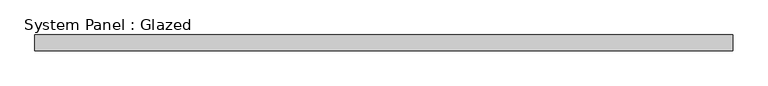
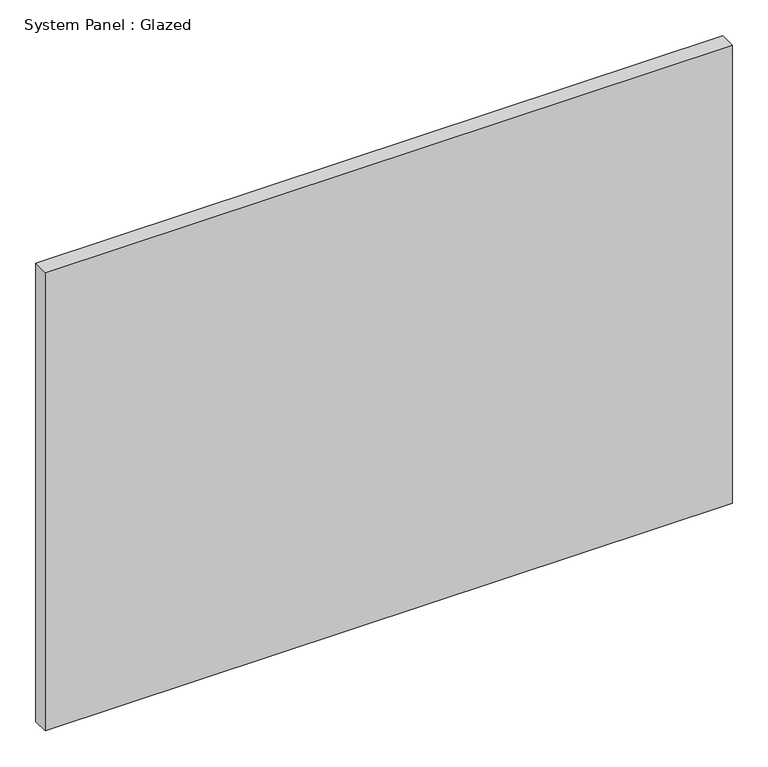
"""IFC4 building model written with IfcOpenShell, lengths in millimetres: plate geometry, System Panel : Glazed."""

from ifc_helpers import new_model, si_unit, origin, origin_with_axes, place, context, project, spatial, polyline, outline, extrude, source, transform, mapped, element, save


def system_panel_glazed_e970100d(model_context):
    return source(origin(), model_context, "Body", "SweptSolid", [
        extrude(outline(polyline([(551.392122, 19.05), (-551.392122, 19.05), (-551.392122, 44.45), (551.392122, 44.45), (551.392122, 19.05)])), origin_with_axes(), (0.0, 0.0, 1.0), 777.5290241),
    ])


if __name__ == "__main__":
    model = new_model("IFC4")
    model_context = context("Model", 3, world=origin())
    ifc_project = project(units=[si_unit("LENGTHUNIT", "METRE", prefix="MILLI")], contexts=[model_context])
    site = spatial("IfcSite", under=ifc_project)
    building = spatial("IfcBuilding", under=site)
    placement = place(None, origin())
    system_panel_glazed_shape = system_panel_glazed_e970100d(model_context)
    element("IfcPlate", 1, ObjectType="System Panel : Glazed", at=placement, inside=building, context=model_context, shape_type="MappedRepresentation", body=[
        mapped(system_panel_glazed_shape, transform((0.0, 0.0, 0.0), x_axis=(1.0, 0.0, 0.0), y_axis=(0.0, 1.0, 0.0), z_axis=(0.0, 0.0, 1.0))),
    ])
    save(model, "model.ifc")

# Revit data of these elements
# Type "System Panel : Glazed"
#   Construction Type Id = "GSP4R"
#   Analytic Construction = "1/8 in Pilkington single glazing"
#   Visual Light Transmittance = 0.9
#   Solar Heat Gain Coefficient = 0.86
#   Heat Transfer Coefficient (U) = 1.18115 BTU/(h·ft²·°F)
# Element 1 (IfcPlate, "System Panel : Glazed")
#   Materials on its faces: "Glass"
# Materials
#   "Glass": class "Glass", colour RGB 0 128 192, transparency 0.75, Description = "Soda Lime Glass", Cost = 0
